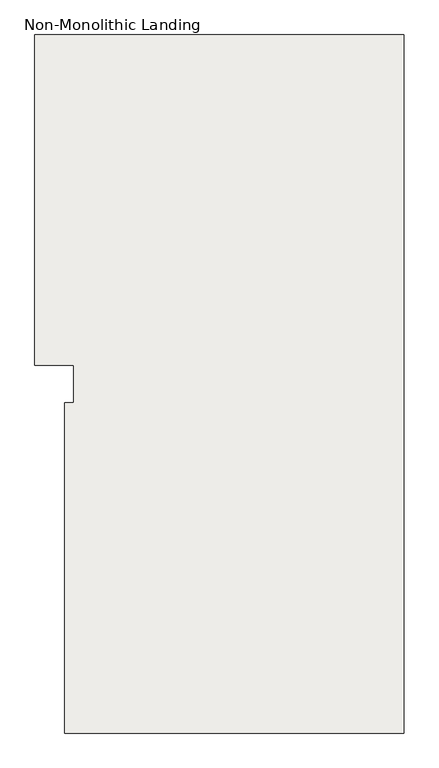
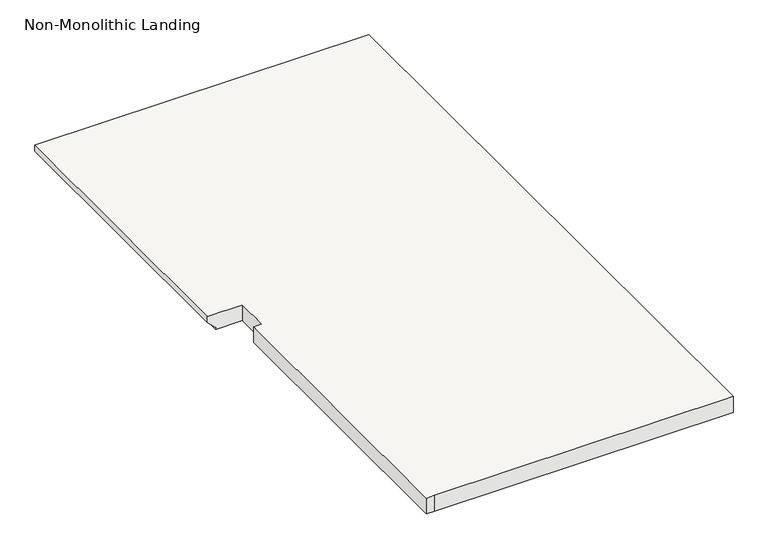
"""IFC4 building model written with IfcOpenShell, lengths in millimetres: slab geometry, Non-Monolithic Landing."""

from ifc_helpers import new_model, si_unit, origin, place, context, project, spatial, faceted_brep, source, transform, mapped, element, save


def non_monolithic_landing_593ffa06(model_context):
    return source(origin(), model_context, "Body", "Brep", [
        faceted_brep([(-5754.9911408, -6224.7337491, 2000.25), (-5754.9911408, -6224.7337491, 2019.3), (-5754.9911408, -5310.3337491, 2019.3), (-5754.9911408, -5310.3337491, 2000.25), (-5729.5911408, -6224.7337491, 1974.85), (-5729.5911408, -5310.3337491, 1974.85), (-5647.5260609, -6224.7337491, 2019.3), (-5647.5260609, -6327.9310793, 2019.3), (-5672.9260609, -6327.9310793, 2019.3), (-5672.9260609, -7242.3310793, 2019.3), (-5647.5260609, -7242.3310793, 2019.3), (-4733.1260609, -7242.3310793, 2019.3), (-4733.1260609, -5310.3337491, 2019.3), (-5729.5911408, -6224.7337491, 1968.5), (-5729.5911408, -5310.3337491, 1968.5), (-4733.1260609, -5310.3337491, 1968.5), (-4733.1260609, -7242.3310793, 1968.5), (-5647.5260609, -7242.3310793, 1968.5), (-5672.9260609, -7242.3310793, 1968.5), (-5672.9260609, -6327.9310793, 1968.5), (-5647.5260609, -6327.9310793, 1968.5), (-5647.5260609, -6224.7337491, 1968.5)], [[[0, 1, 2, 3]], [[4, 0, 3, 5]], [[6, 7, 8, 9, 10, 11, 12, 2, 1]], [[13, 14, 15, 16, 17, 18, 19, 20, 21]], [[14, 13, 4, 5]], [[6, 1, 0, 4, 13, 21]], [[7, 6, 21, 20]], [[8, 7, 20, 19]], [[9, 8, 19, 18]], [[10, 9, 18, 17]], [[11, 10, 17, 16]], [[12, 11, 16, 15]], [[2, 12, 15, 14, 5, 3]]]),
    ])


if __name__ == "__main__":
    model = new_model("IFC4")
    model_context = context("Model", 3, world=origin())
    ifc_project = project(units=[si_unit("LENGTHUNIT", "METRE", prefix="MILLI")], contexts=[model_context])
    site = spatial("IfcSite", under=ifc_project)
    building = spatial("IfcBuilding", under=site)
    placement = place(None, origin())
    non_monolithic_landing_shape = non_monolithic_landing_593ffa06(model_context)
    element("IfcSlab", 1, ObjectType="Non-Monolithic Landing", at=placement, inside=building, context=model_context, shape_type="MappedRepresentation", body=[
        mapped(non_monolithic_landing_shape, transform((0.0, 0.0, 0.0), x_axis=(1.0, 0.0, 0.0), y_axis=(0.0, 1.0, 0.0), z_axis=(0.0, 0.0, 1.0))),
    ])
    save(model, "model.ifc")
